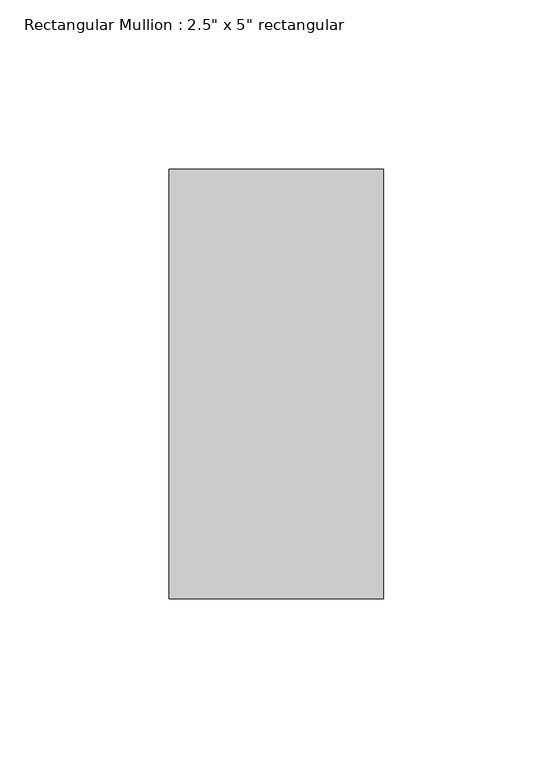
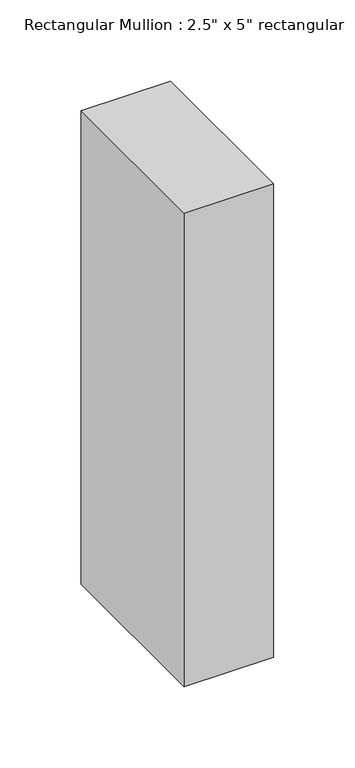
"""IFC4 building model written with IfcOpenShell, lengths in millimetres: member geometry."""

from ifc_helpers import new_model, si_unit, frame, origin, place, context, project, spatial, polyline, outline, extrude, source, transform, mapped, element, save


def member_ca359333(model_context):
    return source(origin(), model_context, "Body", "SweptSolid", [
        extrude(outline(polyline([(31.75, 63.5), (31.75, -63.5), (-31.75, -63.5), (-31.75, 63.5), (31.75, 63.5)])), frame((0.0, 0.0, -355.6), z_axis=(0.0, 0.0, 1.0), x_axis=(1.0, 0.0, 0.0)), (0.0, 0.0, 1.0), 355.6),
    ])


if __name__ == "__main__":
    model = new_model("IFC4")
    model_context = context("Model", 3, world=origin())
    ifc_project = project(units=[si_unit("LENGTHUNIT", "METRE", prefix="MILLI")], contexts=[model_context])
    site = spatial("IfcSite", under=ifc_project)
    building = spatial("IfcBuilding", under=site)
    placement = place(None, origin())
    member_shape = member_ca359333(model_context)
    element("IfcMember", 1, ObjectType="Rectangular Mullion : 2.5\" x 5\" rectangular", at=placement, inside=building, context=model_context, shape_type="MappedRepresentation", body=[
        mapped(member_shape, transform((0.0, 0.0, 0.0), x_axis=(1.0, 0.0, 0.0), y_axis=(0.0, 1.0, 0.0), z_axis=(0.0, 0.0, 1.0))),
    ])
    save(model, "model.ifc")

# Revit data of these elements
# Type "Rectangular Mullion : 2.5\" x 5\" rectangular"
#   built-in parameter 1007304 = 0.416667 (stored number, unit not read)
#   built-in parameter 1007301 = 0.104167 (stored number, unit not read)
#   built-in parameter 1007300 = 0.104167 (stored number, unit not read)
# Element 1 (IfcMember, "Rectangular Mullion : 2.5\" x 5\" rectangular")
#   Materials on its faces: "door colour"
# Materials
#   "door colour": class "Generic", colour RGB 120 120 120, transparency 0, Cost = 0
